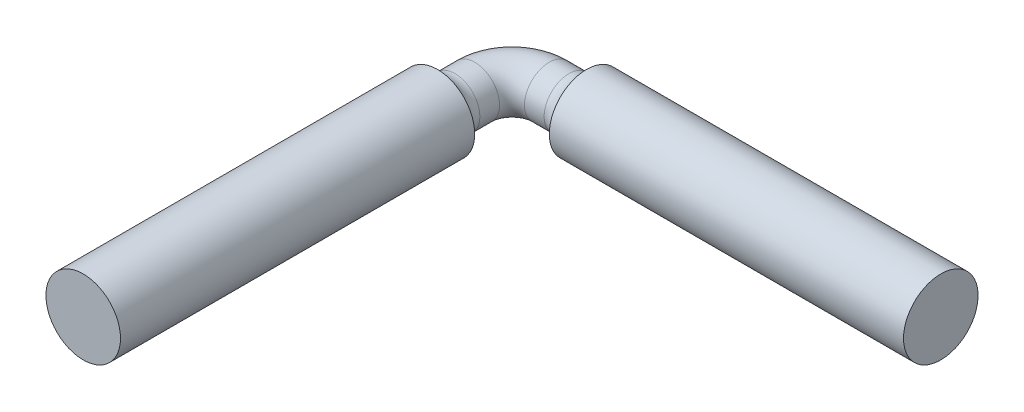
ISO-10303-21;
HEADER;
FILE_DESCRIPTION(('STEP AP214'),'2;1');
FILE_NAME('part.step','',(''),(''),'','','');
FILE_SCHEMA(('AUTOMOTIVE_DESIGN { 1 0 10303 214 1 1 1 1 }'));
ENDSEC;
DATA;
#1=APPLICATION_CONTEXT('core data for automotive mechanical design processes');
#2=APPLICATION_PROTOCOL_DEFINITION('international standard','automotive_design',2000,#1);
#3=PRODUCT_CONTEXT('',#1,'mechanical');
#4=PRODUCT('Part','Part','',(#3));
#5=PRODUCT_RELATED_PRODUCT_CATEGORY('part','',(#4));
#6=PRODUCT_DEFINITION_FORMATION('','',#4);
#7=PRODUCT_DEFINITION_CONTEXT('part definition',#1,'design');
#8=PRODUCT_DEFINITION('design','',#6,#7);
#9=PRODUCT_DEFINITION_SHAPE('','',#8);
#10=(LENGTH_UNIT() NAMED_UNIT(*) SI_UNIT(.MILLI.,.METRE.));
#11=(NAMED_UNIT(*) PLANE_ANGLE_UNIT() SI_UNIT($,.RADIAN.));
#12=(NAMED_UNIT(*) SI_UNIT($,.STERADIAN.) SOLID_ANGLE_UNIT());
#13=UNCERTAINTY_MEASURE_WITH_UNIT(LENGTH_MEASURE(1.E-05),#10,'distance_accuracy_value','');
#14=(GEOMETRIC_REPRESENTATION_CONTEXT(3) GLOBAL_UNCERTAINTY_ASSIGNED_CONTEXT((#13)) GLOBAL_UNIT_ASSIGNED_CONTEXT((#10,
#11,#12)) REPRESENTATION_CONTEXT('',''));
#15=CARTESIAN_POINT('',(0.,0.,0.));
#16=DIRECTION('',(0.,0.,1.));
#17=DIRECTION('',(1.,0.,0.));
#18=AXIS2_PLACEMENT_3D('',#15,#16,#17);
#19=CARTESIAN_POINT('',(0.,0.,-28.5));
#20=DIRECTION('',(0.,0.,1.));
#21=DIRECTION('',(1.,0.,0.));
#22=AXIS2_PLACEMENT_3D('',#19,#20,#21);
#23=CYLINDRICAL_SURFACE('',#22,3.);
#24=CARTESIAN_POINT('',(0.,0.,-28.5));
#25=DIRECTION('',(0.,0.,1.));
#26=DIRECTION('',(1.,0.,0.));
#27=AXIS2_PLACEMENT_3D('',#24,#25,#26);
#28=CIRCLE('',#27,3.);
#29=CARTESIAN_POINT('',(3.,0.,-28.5));
#30=VERTEX_POINT('',#29);
#31=EDGE_CURVE('E58',#30,#30,#28,.T.);
#32=CARTESIAN_POINT('',(0.,0.,0.));
#33=DIRECTION('',(0.,0.,1.));
#34=DIRECTION('',(1.,0.,0.));
#35=AXIS2_PLACEMENT_3D('',#32,#33,#34);
#36=CIRCLE('',#35,3.);
#37=CARTESIAN_POINT('',(3.,0.,0.));
#38=VERTEX_POINT('',#37);
#39=EDGE_CURVE('E61',#38,#38,#36,.T.);
#40=CARTESIAN_POINT('',(3.,0.,-28.5));
#41=CARTESIAN_POINT('',(3.,0.,-28.203125));
#42=CARTESIAN_POINT('',(3.,0.,-27.90625));
#43=CARTESIAN_POINT('',(3.,0.,-27.3125));
#44=CARTESIAN_POINT('',(3.,0.,-27.015625));
#45=CARTESIAN_POINT('',(3.,0.,-26.421875));
#46=CARTESIAN_POINT('',(3.,0.,-26.125));
#47=CARTESIAN_POINT('',(3.,0.,-25.53125));
#48=CARTESIAN_POINT('',(3.,0.,-25.234375));
#49=CARTESIAN_POINT('',(3.,0.,-24.640625));
#50=CARTESIAN_POINT('',(3.,0.,-24.34375));
#51=CARTESIAN_POINT('',(3.,0.,-23.75));
#52=CARTESIAN_POINT('',(3.,0.,-23.453125));
#53=CARTESIAN_POINT('',(3.,0.,-22.859375));
#54=CARTESIAN_POINT('',(3.,0.,-22.5625));
#55=CARTESIAN_POINT('',(3.,0.,-21.96875));
#56=CARTESIAN_POINT('',(3.,0.,-21.671875));
#57=CARTESIAN_POINT('',(3.,0.,-21.078125));
#58=CARTESIAN_POINT('',(3.,0.,-20.78125));
#59=CARTESIAN_POINT('',(3.,0.,-20.1875));
#60=CARTESIAN_POINT('',(3.,0.,-19.890625));
#61=CARTESIAN_POINT('',(3.,0.,-19.296875));
#62=CARTESIAN_POINT('',(3.,0.,-19.));
#63=CARTESIAN_POINT('',(3.,0.,-18.40625));
#64=CARTESIAN_POINT('',(3.,0.,-18.109375));
#65=CARTESIAN_POINT('',(3.,0.,-17.515625));
#66=CARTESIAN_POINT('',(3.,0.,-17.21875));
#67=CARTESIAN_POINT('',(3.,0.,-16.625));
#68=CARTESIAN_POINT('',(3.,0.,-16.328125));
#69=CARTESIAN_POINT('',(3.,0.,-15.734375));
#70=CARTESIAN_POINT('',(3.,0.,-15.4375));
#71=CARTESIAN_POINT('',(3.,0.,-14.84375));
#72=CARTESIAN_POINT('',(3.,0.,-14.546875));
#73=CARTESIAN_POINT('',(3.,0.,-13.953125));
#74=CARTESIAN_POINT('',(3.,0.,-13.65625));
#75=CARTESIAN_POINT('',(3.,0.,-13.0625));
#76=CARTESIAN_POINT('',(3.,0.,-12.765625));
#77=CARTESIAN_POINT('',(3.,0.,-12.171875));
#78=CARTESIAN_POINT('',(3.,0.,-11.875));
#79=CARTESIAN_POINT('',(3.,0.,-11.28125));
#80=CARTESIAN_POINT('',(3.,0.,-10.984375));
#81=CARTESIAN_POINT('',(3.,0.,-10.390625));
#82=CARTESIAN_POINT('',(3.,0.,-10.09375));
#83=CARTESIAN_POINT('',(3.,0.,-9.5));
#84=CARTESIAN_POINT('',(3.,0.,-9.203125));
#85=CARTESIAN_POINT('',(3.,0.,-8.609375));
#86=CARTESIAN_POINT('',(3.,0.,-8.3125));
#87=CARTESIAN_POINT('',(3.,0.,-7.71875));
#88=CARTESIAN_POINT('',(3.,0.,-7.421875));
#89=CARTESIAN_POINT('',(3.,0.,-6.828125));
#90=CARTESIAN_POINT('',(3.,0.,-6.53125));
#91=CARTESIAN_POINT('',(3.,0.,-5.9375));
#92=CARTESIAN_POINT('',(3.,0.,-5.640625));
#93=CARTESIAN_POINT('',(3.,0.,-5.046875));
#94=CARTESIAN_POINT('',(3.,0.,-4.75));
#95=CARTESIAN_POINT('',(3.,0.,-4.15625));
#96=CARTESIAN_POINT('',(3.,0.,-3.859375));
#97=CARTESIAN_POINT('',(3.,0.,-3.265625));
#98=CARTESIAN_POINT('',(3.,0.,-2.96875));
#99=CARTESIAN_POINT('',(3.,0.,-2.375));
#100=CARTESIAN_POINT('',(3.,0.,-2.078125));
#101=CARTESIAN_POINT('',(3.,0.,-1.484375));
#102=CARTESIAN_POINT('',(3.,0.,-1.1875));
#103=CARTESIAN_POINT('',(3.,0.,-0.593749999999999));
#104=CARTESIAN_POINT('',(3.,0.,-0.296875));
#105=CARTESIAN_POINT('',(3.,0.,0.));
#106=B_SPLINE_CURVE_WITH_KNOTS('',3,(#40,#41,#42,#43,#44,#45,#46,#47,#48,#49,#50,#51,#52,#53,
#54,#55,#56,#57,#58,#59,#60,#61,#62,#63,#64,#65,#66,#67,#68,#69,#70,#71,#72,#73,#74,#75,#76,#77,
#78,#79,#80,#81,#82,#83,#84,#85,#86,#87,#88,#89,#90,#91,#92,#93,#94,#95,#96,#97,#98,#99,#100,
#101,#102,#103,#104,#105),.UNSPECIFIED.,.F.,.F.,(4,2,2,2,2,2,2,2,2,2,2,2,2,2,2,2,2,2,2,2,2,2,2,
2,2,2,2,2,2,2,2,2,4),(0.,0.890624999999999,1.78125,2.671875,3.5625,4.453125,5.34375,6.234375,
7.125,8.015625,8.90625,9.796875,10.6875,11.578125,12.46875,13.359375,14.25,15.140625,16.03125,
16.921875,17.8125,18.703125,19.59375,20.484375,21.375,22.265625,23.15625,24.046875,24.9375,
25.828125,26.71875,27.609375,28.5),.UNSPECIFIED.);
#107=EDGE_CURVE('BSEAM47',#30,#38,#106,.T.);
#108=ORIENTED_EDGE('',*,*,#31,.T.);
#109=ORIENTED_EDGE('',*,*,#39,.F.);
#110=ORIENTED_EDGE('',*,*,#107,.T.);
#111=ORIENTED_EDGE('',*,*,#107,.F.);
#112=EDGE_LOOP('',(#108,#110,#109,#111));
#113=FACE_BOUND('',#112,.T.);
#114=ADVANCED_FACE('F47',(#113),#23,.T.);
#115=CARTESIAN_POINT('',(0.,0.,0.));
#116=DIRECTION('',(0.,0.,1.));
#117=DIRECTION('',(1.,0.,0.));
#118=AXIS2_PLACEMENT_3D('',#115,#116,#117);
#119=PLANE('',#118);
#120=ORIENTED_EDGE('',*,*,#39,.T.);
#121=EDGE_LOOP('',(#120));
#122=FACE_BOUND('',#121,.T.);
#123=ADVANCED_FACE('F102',(#122),#119,.T.);
#124=CARTESIAN_POINT('',(0.,0.,-28.5));
#125=DIRECTION('',(0.,0.,-1.));
#126=DIRECTION('',(-1.,0.,0.));
#127=AXIS2_PLACEMENT_3D('',#124,#125,#126);
#128=CYLINDRICAL_SURFACE('',#127,2.);
#129=CARTESIAN_POINT('',(0.,0.,-29.9142135623731));
#130=DIRECTION('',(0.,0.,1.));
#131=DIRECTION('',(1.,0.,0.));
#132=AXIS2_PLACEMENT_3D('',#129,#130,#131);
#133=CIRCLE('',#132,2.);
#134=CARTESIAN_POINT('',(2.,0.,-29.9142135623731));
#135=VERTEX_POINT('',#134);
#136=EDGE_CURVE('E11',#135,#135,#133,.F.);
#137=ORIENTED_EDGE('',*,*,#136,.T.);
#138=EDGE_LOOP('',(#137));
#139=FACE_BOUND('',#138,.T.);
#140=CARTESIAN_POINT('',(0.,0.,-31.5));
#141=DIRECTION('',(0.,0.,1.));
#142=DIRECTION('',(1.,0.,0.));
#143=AXIS2_PLACEMENT_3D('',#140,#141,#142);
#144=CIRCLE('',#143,2.);
#145=CARTESIAN_POINT('',(-2.,0.,-31.5));
#146=VERTEX_POINT('',#145);
#147=EDGE_CURVE('E75',#146,#146,#144,.T.);
#148=ORIENTED_EDGE('',*,*,#147,.T.);
#149=EDGE_LOOP('',(#148));
#150=FACE_BOUND('',#149,.T.);
#151=ADVANCED_FACE('F86',(#139,#150),#128,.T.);
#152=CARTESIAN_POINT('',(3.,0.,-31.5));
#153=DIRECTION('',(0.,-1.,0.));
#154=DIRECTION('',(0.,0.,-1.));
#155=AXIS2_PLACEMENT_3D('',#152,#153,#154);
#156=TOROIDAL_SURFACE('',#155,3.,2.);
#157=CARTESIAN_POINT('',(3.,0.,-34.5));
#158=DIRECTION('',(-1.,0.,0.));
#159=DIRECTION('',(0.,0.,1.));
#160=AXIS2_PLACEMENT_3D('',#157,#158,#159);
#161=CIRCLE('',#160,2.);
#162=CARTESIAN_POINT('',(3.,0.,-36.5));
#163=VERTEX_POINT('',#162);
#164=EDGE_CURVE('E69',#163,#163,#161,.T.);
#165=CARTESIAN_POINT('',(3.,0.,-31.5));
#166=DIRECTION('',(0.,-1.,0.));
#167=DIRECTION('',(0.,0.,-1.));
#168=AXIS2_PLACEMENT_3D('',#165,#166,#167);
#169=CIRCLE('',#168,5.);
#170=EDGE_CURVE('',#146,#163,#169,.T.);
#171=ORIENTED_EDGE('',*,*,#147,.F.);
#172=ORIENTED_EDGE('',*,*,#164,.T.);
#173=ORIENTED_EDGE('',*,*,#170,.T.);
#174=ORIENTED_EDGE('',*,*,#170,.F.);
#175=EDGE_LOOP('',(#171,#173,#172,#174));
#176=FACE_BOUND('',#175,.T.);
#177=ADVANCED_FACE('F114',(#176),#156,.T.);
#178=CARTESIAN_POINT('',(3.,0.,-34.5));
#179=DIRECTION('',(1.,0.,0.));
#180=DIRECTION('',(0.,0.,-1.));
#181=AXIS2_PLACEMENT_3D('',#178,#179,#180);
#182=CYLINDRICAL_SURFACE('',#181,2.);
#183=CARTESIAN_POINT('',(4.5857864376269,0.,-34.5));
#184=DIRECTION('',(1.,0.,0.));
#185=DIRECTION('',(0.,0.,-1.));
#186=AXIS2_PLACEMENT_3D('',#183,#184,#185);
#187=CIRCLE('',#186,2.);
#188=CARTESIAN_POINT('',(4.5857864376269,0.,-36.5));
#189=VERTEX_POINT('',#188);
#190=EDGE_CURVE('E57',#189,#189,#187,.F.);
#191=CARTESIAN_POINT('',(4.5857864376269,0.,-36.5));
#192=CARTESIAN_POINT('',(4.56926782890162,0.,-36.5));
#193=CARTESIAN_POINT('',(4.55274922017634,0.,-36.5));
#194=CARTESIAN_POINT('',(4.51971200272578,0.,-36.5));
#195=CARTESIAN_POINT('',(4.5031933940005,0.,-36.5));
#196=CARTESIAN_POINT('',(4.47015617654994,0.,-36.5));
#197=CARTESIAN_POINT('',(4.45363756782466,0.,-36.5));
#198=CARTESIAN_POINT('',(4.4206003503741,0.,-36.5));
#199=CARTESIAN_POINT('',(4.40408174164882,0.,-36.5));
#200=CARTESIAN_POINT('',(4.37104452419826,0.,-36.5));
#201=CARTESIAN_POINT('',(4.35452591547298,0.,-36.5));
#202=CARTESIAN_POINT('',(4.32148869802242,0.,-36.5));
#203=CARTESIAN_POINT('',(4.30497008929714,0.,-36.5));
#204=CARTESIAN_POINT('',(4.27193287184658,0.,-36.5));
#205=CARTESIAN_POINT('',(4.2554142631213,0.,-36.5));
#206=CARTESIAN_POINT('',(4.22237704567074,0.,-36.5));
#207=CARTESIAN_POINT('',(4.20585843694546,0.,-36.5));
#208=CARTESIAN_POINT('',(4.1728212194949,0.,-36.5));
#209=CARTESIAN_POINT('',(4.15630261076962,0.,-36.5));
#210=CARTESIAN_POINT('',(4.12326539331906,0.,-36.5));
#211=CARTESIAN_POINT('',(4.10674678459378,0.,-36.5));
#212=CARTESIAN_POINT('',(4.07370956714322,0.,-36.5));
#213=CARTESIAN_POINT('',(4.05719095841793,0.,-36.5));
#214=CARTESIAN_POINT('',(4.02415374096737,0.,-36.5));
#215=CARTESIAN_POINT('',(4.0076351322421,0.,-36.5));
#216=CARTESIAN_POINT('',(3.97459791479153,0.,-36.5));
#217=CARTESIAN_POINT('',(3.95807930606625,0.,-36.5));
#218=CARTESIAN_POINT('',(3.92504208861569,0.,-36.5));
#219=CARTESIAN_POINT('',(3.90852347989041,0.,-36.5));
#220=CARTESIAN_POINT('',(3.87548626243985,0.,-36.5));
#221=CARTESIAN_POINT('',(3.85896765371457,0.,-36.5));
#222=CARTESIAN_POINT('',(3.82593043626401,0.,-36.5));
#223=CARTESIAN_POINT('',(3.80941182753873,0.,-36.5));
#224=CARTESIAN_POINT('',(3.77637461008817,0.,-36.5));
#225=CARTESIAN_POINT('',(3.75985600136289,0.,-36.5));
#226=CARTESIAN_POINT('',(3.72681878391233,0.,-36.5));
#227=CARTESIAN_POINT('',(3.71030017518705,0.,-36.5));
#228=CARTESIAN_POINT('',(3.67726295773649,0.,-36.5));
#229=CARTESIAN_POINT('',(3.66074434901121,0.,-36.5));
#230=CARTESIAN_POINT('',(3.62770713156065,0.,-36.5));
#231=CARTESIAN_POINT('',(3.61118852283537,0.,-36.5));
#232=CARTESIAN_POINT('',(3.57815130538481,0.,-36.5));
#233=CARTESIAN_POINT('',(3.56163269665953,0.,-36.5));
#234=CARTESIAN_POINT('',(3.52859547920897,0.,-36.5));
#235=CARTESIAN_POINT('',(3.51207687048369,0.,-36.5));
#236=CARTESIAN_POINT('',(3.47903965303313,0.,-36.5));
#237=CARTESIAN_POINT('',(3.46252104430785,0.,-36.5));
#238=CARTESIAN_POINT('',(3.42948382685729,0.,-36.5));
#239=CARTESIAN_POINT('',(3.41296521813201,0.,-36.5));
#240=CARTESIAN_POINT('',(3.37992800068145,0.,-36.5));
#241=CARTESIAN_POINT('',(3.36340939195616,0.,-36.5));
#242=CARTESIAN_POINT('',(3.3303721745056,0.,-36.5));
#243=CARTESIAN_POINT('',(3.31385356578032,0.,-36.5));
#244=CARTESIAN_POINT('',(3.28081634832976,0.,-36.5));
#245=CARTESIAN_POINT('',(3.26429773960448,0.,-36.5));
#246=CARTESIAN_POINT('',(3.23126052215392,0.,-36.5));
#247=CARTESIAN_POINT('',(3.21474191342864,0.,-36.5));
#248=CARTESIAN_POINT('',(3.18170469597808,0.,-36.5));
#249=CARTESIAN_POINT('',(3.1651860872528,0.,-36.5));
#250=CARTESIAN_POINT('',(3.13214886980224,0.,-36.5));
#251=CARTESIAN_POINT('',(3.11563026107696,0.,-36.5));
#252=CARTESIAN_POINT('',(3.0825930436264,0.,-36.5));
#253=CARTESIAN_POINT('',(3.06607443490112,0.,-36.5));
#254=CARTESIAN_POINT('',(3.03303721745056,0.,-36.5));
#255=CARTESIAN_POINT('',(3.01651860872528,0.,-36.5));
#256=CARTESIAN_POINT('',(3.,0.,-36.5));
#257=B_SPLINE_CURVE_WITH_KNOTS('',3,(#191,#192,#193,#194,#195,#196,#197,#198,#199,#200,#201,
#202,#203,#204,#205,#206,#207,#208,#209,#210,#211,#212,#213,#214,#215,#216,#217,#218,#219,#220,
#221,#222,#223,#224,#225,#226,#227,#228,#229,#230,#231,#232,#233,#234,#235,#236,#237,#238,#239,
#240,#241,#242,#243,#244,#245,#246,#247,#248,#249,#250,#251,#252,#253,#254,#255,#256),
.UNSPECIFIED.,.F.,.F.,(4,2,2,2,2,2,2,2,2,2,2,2,2,2,2,2,2,2,2,2,2,2,2,2,2,2,2,2,2,2,2,2,4),(0.,
0.0495558261758402,0.0991116523516812,0.148667478527522,0.198223304703362,0.247779130879203,
0.297334957055044,0.346890783230885,0.396446609406726,0.446002435582567,0.495558261758407,
0.545114087934248,0.594669914110088,0.644225740285929,0.69378156646177,0.743337392637611,
0.792893218813451,0.842449044989292,0.892004871165132,0.941560697340973,0.991116523516814,
1.04067234969265,1.0902281758685,1.13978400204434,1.18933982822018,1.23889565439602,
1.28845148057186,1.3380073067477,1.38756313292354,1.43711895909938,1.48667478527522,
1.53623061145106,1.5857864376269),.UNSPECIFIED.);
#258=EDGE_CURVE('BSEAM90',#189,#163,#257,.T.);
#259=ORIENTED_EDGE('',*,*,#190,.T.);
#260=ORIENTED_EDGE('',*,*,#164,.F.);
#261=ORIENTED_EDGE('',*,*,#258,.T.);
#262=ORIENTED_EDGE('',*,*,#258,.F.);
#263=EDGE_LOOP('',(#259,#261,#260,#262));
#264=FACE_BOUND('',#263,.T.);
#265=ADVANCED_FACE('F90',(#264),#182,.T.);
#266=CARTESIAN_POINT('',(34.5,0.,-34.5));
#267=DIRECTION('',(-1.,0.,0.));
#268=DIRECTION('',(0.,0.,1.));
#269=AXIS2_PLACEMENT_3D('',#266,#267,#268);
#270=CYLINDRICAL_SURFACE('',#269,3.);
#271=CARTESIAN_POINT('',(34.5,0.,-34.5));
#272=DIRECTION('',(1.,0.,0.));
#273=DIRECTION('',(0.,0.,-1.));
#274=AXIS2_PLACEMENT_3D('',#271,#272,#273);
#275=CIRCLE('',#274,3.);
#276=CARTESIAN_POINT('',(34.5,0.,-31.5));
#277=VERTEX_POINT('',#276);
#278=EDGE_CURVE('E74',#277,#277,#275,.T.);
#279=CARTESIAN_POINT('',(6.,0.,-34.5));
#280=DIRECTION('',(1.,0.,0.));
#281=DIRECTION('',(0.,0.,-1.));
#282=AXIS2_PLACEMENT_3D('',#279,#280,#281);
#283=CIRCLE('',#282,3.);
#284=CARTESIAN_POINT('',(6.,0.,-31.5));
#285=VERTEX_POINT('',#284);
#286=EDGE_CURVE('E77',#285,#285,#283,.T.);
#287=CARTESIAN_POINT('',(34.5,0.,-31.5));
#288=CARTESIAN_POINT('',(34.203125,0.,-31.5));
#289=CARTESIAN_POINT('',(33.90625,0.,-31.5));
#290=CARTESIAN_POINT('',(33.3125,0.,-31.5));
#291=CARTESIAN_POINT('',(33.015625,0.,-31.5));
#292=CARTESIAN_POINT('',(32.421875,0.,-31.5));
#293=CARTESIAN_POINT('',(32.125,0.,-31.5));
#294=CARTESIAN_POINT('',(31.53125,0.,-31.5));
#295=CARTESIAN_POINT('',(31.234375,0.,-31.5));
#296=CARTESIAN_POINT('',(30.640625,0.,-31.5));
#297=CARTESIAN_POINT('',(30.34375,0.,-31.5));
#298=CARTESIAN_POINT('',(29.75,0.,-31.5));
#299=CARTESIAN_POINT('',(29.453125,0.,-31.5));
#300=CARTESIAN_POINT('',(28.859375,0.,-31.5));
#301=CARTESIAN_POINT('',(28.5625,0.,-31.5));
#302=CARTESIAN_POINT('',(27.96875,0.,-31.5));
#303=CARTESIAN_POINT('',(27.671875,0.,-31.5));
#304=CARTESIAN_POINT('',(27.078125,0.,-31.5));
#305=CARTESIAN_POINT('',(26.78125,0.,-31.5));
#306=CARTESIAN_POINT('',(26.1875,0.,-31.5));
#307=CARTESIAN_POINT('',(25.890625,0.,-31.5));
#308=CARTESIAN_POINT('',(25.296875,0.,-31.5));
#309=CARTESIAN_POINT('',(25.,0.,-31.5));
#310=CARTESIAN_POINT('',(24.40625,0.,-31.5));
#311=CARTESIAN_POINT('',(24.109375,0.,-31.5));
#312=CARTESIAN_POINT('',(23.515625,0.,-31.5));
#313=CARTESIAN_POINT('',(23.21875,0.,-31.5));
#314=CARTESIAN_POINT('',(22.625,0.,-31.5));
#315=CARTESIAN_POINT('',(22.328125,0.,-31.5));
#316=CARTESIAN_POINT('',(21.734375,0.,-31.5));
#317=CARTESIAN_POINT('',(21.4375,0.,-31.5));
#318=CARTESIAN_POINT('',(20.84375,0.,-31.5));
#319=CARTESIAN_POINT('',(20.546875,0.,-31.5));
#320=CARTESIAN_POINT('',(19.953125,0.,-31.5));
#321=CARTESIAN_POINT('',(19.65625,0.,-31.5));
#322=CARTESIAN_POINT('',(19.0625,0.,-31.5));
#323=CARTESIAN_POINT('',(18.765625,0.,-31.5));
#324=CARTESIAN_POINT('',(18.171875,0.,-31.5));
#325=CARTESIAN_POINT('',(17.875,0.,-31.5));
#326=CARTESIAN_POINT('',(17.28125,0.,-31.5));
#327=CARTESIAN_POINT('',(16.984375,0.,-31.5));
#328=CARTESIAN_POINT('',(16.390625,0.,-31.5));
#329=CARTESIAN_POINT('',(16.09375,0.,-31.5));
#330=CARTESIAN_POINT('',(15.5,0.,-31.5));
#331=CARTESIAN_POINT('',(15.203125,0.,-31.5));
#332=CARTESIAN_POINT('',(14.609375,0.,-31.5));
#333=CARTESIAN_POINT('',(14.3125,0.,-31.5));
#334=CARTESIAN_POINT('',(13.71875,0.,-31.5));
#335=CARTESIAN_POINT('',(13.421875,0.,-31.5));
#336=CARTESIAN_POINT('',(12.828125,0.,-31.5));
#337=CARTESIAN_POINT('',(12.53125,0.,-31.5));
#338=CARTESIAN_POINT('',(11.9375,0.,-31.5));
#339=CARTESIAN_POINT('',(11.640625,0.,-31.5));
#340=CARTESIAN_POINT('',(11.046875,0.,-31.5));
#341=CARTESIAN_POINT('',(10.75,0.,-31.5));
#342=CARTESIAN_POINT('',(10.15625,0.,-31.5));
#343=CARTESIAN_POINT('',(9.859375,0.,-31.5));
#344=CARTESIAN_POINT('',(9.265625,0.,-31.5));
#345=CARTESIAN_POINT('',(8.96875,0.,-31.5));
#346=CARTESIAN_POINT('',(8.375,0.,-31.5));
#347=CARTESIAN_POINT('',(8.078125,0.,-31.5));
#348=CARTESIAN_POINT('',(7.484375,0.,-31.5));
#349=CARTESIAN_POINT('',(7.1875,0.,-31.5));
#350=CARTESIAN_POINT('',(6.59375,0.,-31.5));
#351=CARTESIAN_POINT('',(6.296875,0.,-31.5));
#352=CARTESIAN_POINT('',(6.,0.,-31.5));
#353=B_SPLINE_CURVE_WITH_KNOTS('',3,(#287,#288,#289,#290,#291,#292,#293,#294,#295,#296,#297,
#298,#299,#300,#301,#302,#303,#304,#305,#306,#307,#308,#309,#310,#311,#312,#313,#314,#315,#316,
#317,#318,#319,#320,#321,#322,#323,#324,#325,#326,#327,#328,#329,#330,#331,#332,#333,#334,#335,
#336,#337,#338,#339,#340,#341,#342,#343,#344,#345,#346,#347,#348,#349,#350,#351,#352),
.UNSPECIFIED.,.F.,.F.,(4,2,2,2,2,2,2,2,2,2,2,2,2,2,2,2,2,2,2,2,2,2,2,2,2,2,2,2,2,2,2,2,4),(0.,
0.890624999999999,1.78125,2.671875,3.5625,4.453125,5.34374999999999,6.234375,7.125,
8.01562499999999,8.90625,9.796875,10.6875,11.578125,12.46875,13.359375,14.25,15.140625,16.03125,
16.921875,17.8125,18.703125,19.59375,20.484375,21.375,22.265625,23.15625,24.046875,24.9375,
25.828125,26.71875,27.609375,28.5),.UNSPECIFIED.);
#354=EDGE_CURVE('BSEAM81',#277,#285,#353,.T.);
#355=ORIENTED_EDGE('',*,*,#278,.F.);
#356=ORIENTED_EDGE('',*,*,#286,.T.);
#357=ORIENTED_EDGE('',*,*,#354,.T.);
#358=ORIENTED_EDGE('',*,*,#354,.F.);
#359=EDGE_LOOP('',(#355,#357,#356,#358));
#360=FACE_BOUND('',#359,.T.);
#361=ADVANCED_FACE('F81',(#360),#270,.T.);
#362=CARTESIAN_POINT('',(34.5,0.,-34.5));
#363=DIRECTION('',(1.,0.,0.));
#364=DIRECTION('',(0.,0.,-1.));
#365=AXIS2_PLACEMENT_3D('',#362,#363,#364);
#366=PLANE('',#365);
#367=ORIENTED_EDGE('',*,*,#278,.T.);
#368=EDGE_LOOP('',(#367));
#369=FACE_BOUND('',#368,.T.);
#370=ADVANCED_FACE('F85',(#369),#366,.T.);
#371=CARTESIAN_POINT('',(4.5857864376269,0.,-34.5));
#372=DIRECTION('',(1.,0.,0.));
#373=DIRECTION('',(0.,0.,-1.));
#374=AXIS2_PLACEMENT_3D('',#371,#372,#373);
#375=TOROIDAL_SURFACE('',#374,3.5,1.5);
#376=ORIENTED_EDGE('',*,*,#286,.F.);
#377=EDGE_LOOP('',(#376));
#378=FACE_BOUND('',#377,.T.);
#379=ORIENTED_EDGE('',*,*,#190,.F.);
#380=EDGE_LOOP('',(#379));
#381=FACE_BOUND('',#380,.T.);
#382=ADVANCED_FACE('F95',(#378,#381),#375,.F.);
#383=CARTESIAN_POINT('',(0.,0.,-29.9142135623731));
#384=DIRECTION('',(0.,0.,1.));
#385=DIRECTION('',(1.,0.,0.));
#386=AXIS2_PLACEMENT_3D('',#383,#384,#385);
#387=TOROIDAL_SURFACE('',#386,3.5,1.5);
#388=ORIENTED_EDGE('',*,*,#136,.F.);
#389=EDGE_LOOP('',(#388));
#390=FACE_BOUND('',#389,.T.);
#391=ORIENTED_EDGE('',*,*,#31,.F.);
#392=EDGE_LOOP('',(#391));
#393=FACE_BOUND('',#392,.T.);
#394=ADVANCED_FACE('F51',(#390,#393),#387,.F.);
#395=CLOSED_SHELL('',(#114,#123,#151,#177,#265,#361,#370,#382,#394));
#396=MANIFOLD_SOLID_BREP('B2',#395);
#397=ADVANCED_BREP_SHAPE_REPRESENTATION('',(#18,#396),#14);
#398=SHAPE_DEFINITION_REPRESENTATION(#9,#397);
ENDSEC;
END-ISO-10303-21;
